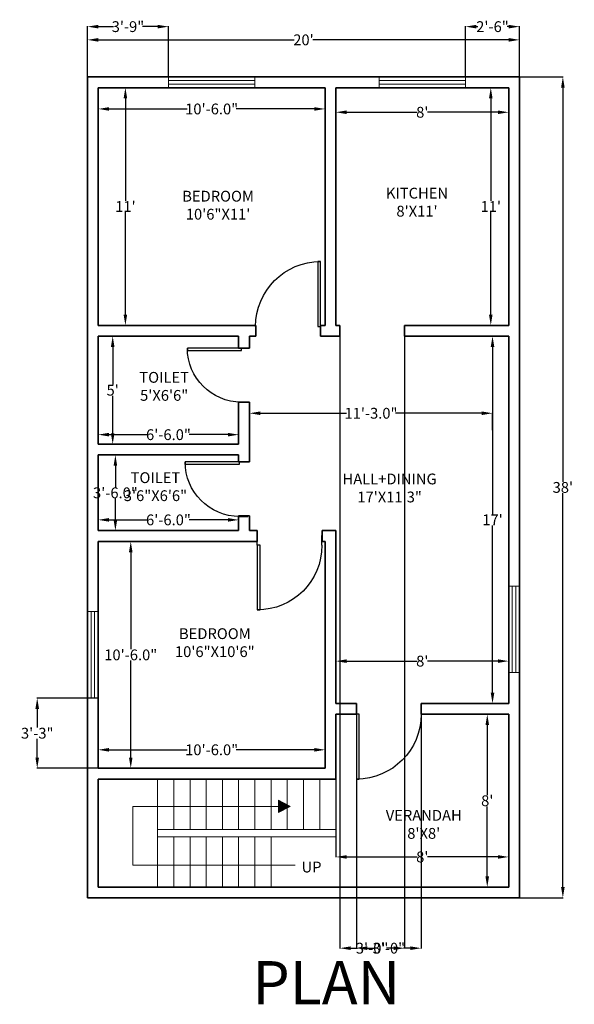
# Model space of a CAD drawing. Units: inches. Extents: x 329 to 1300, y 173 to 760.
# Tile 1 of 3: x 329 to 637, y 214 to 760. Entities that reach past the tile are written whole.
import ezdxf

# ---------------------------------------------------------------- set-up
doc = ezdxf.new("R2010")
doc.units = ezdxf.units.IN
doc.header["$MEASUREMENT"] = 0
doc.layers.add('A-ANNO-PATT', color=251, linetype='Continuous', lineweight=13, true_color=0x636466)
for name, color, linetype, lineweight in [('A-ANNO-SYMB', 7, 'Continuous', 18), ('A-ANNO-TEXT', 7, 'Continuous', 18), ('A-ANNO-TITL', 1, 'Continuous', 25), ('A-AREA-IDEN', 1, 'Continuous', 18), ('A-FLOR-STRS', 7, 'Continuous', 18), ('A-GLAZ', 4, 'Continuous', 18), ('A-WALL', 7, 'Continuous', 35), ('DIMENSION', 80, 'Continuous', 13), ('DOOR', 27, 'Continuous', 25)]:
    doc.layers.add(name, color=color, linetype=linetype, lineweight=lineweight)
doc.styles.get("Standard").update_dxf_attribs({"font": 'arial.ttf'})
doc.dimstyles.get("Standard").update_dxf_attribs({"dimtxt": 6, "dimasz": 6, "dimexe": 0.18, "dimexo": 0.0625, "dimgap": 0.09, "dimtad": 0, "dimtih": 1, "dimtoh": 1, "dimdec": 1, "dimzin": 0, "dimdsep": 46, "dimlunit": 3, "dimtxsty": 'Standard', "dimcen": 0.09, "dimadec": 0, "dimazin": 0, "dimtfac": 1, "dimtdec": 1, "dimtofl": 0, "dimtmove": 0, "dimatfit": 3, "dimfxl": 1, "dimtolj": 1, "dimtzin": 0, "dimarcsym": 0})

# ---------------------------------------------------------------- blocks, each defined once
blk = doc.blocks.new('*U2')
for p, q in [((0, 0), (0, -6)), ((40, 0), (40, -6))]:
    blk.add_line(p, q)
blk.add_lwpolyline([(0, 0), (0, 40), (1.75, 40), (1.75, 0)], close=True)
blk.add_arc((0, 0), 40, 0, 90)
blk = doc.blocks.new('*D22')
at = {"layer": 'Defpoints', "color": 0, "transparency": 16777216}
for p in [(606.67, 749.18), (366.67, 728.62), (606.67, 728.62)]:
    blk.add_point(p, dxfattribs=at)
at = {"layer": 'DIMENSION', "color": 0, "lineweight": -2, "transparency": 16777216}
for p, q in [((366.67, 728.68), (366.67, 749.36)), ((372.67, 749.18), (481.44, 749.18)), ((600.67, 749.18), (491.9, 749.18)), ((606.67, 728.68), (606.67, 749.36))]:
    blk.add_line(p, q, dxfattribs=at)
at = {"layer": 'DIMENSION', "color": 0, "transparency": 16777216}
for points in [[(372.67, 750.18), (372.67, 748.18), (366.67, 749.18)], [(600.67, 750.18), (600.67, 748.18), (606.67, 749.18)]]:
    blk.add_solid(points, dxfattribs=at)
at = {"layer": 'DIMENSION', "color": 0, "transparency": 16777216, "insert": (486.67, 749.18), "char_height": 6, "attachment_point": 5}
blk.add_mtext("\\A1;20'", dxfattribs=at)
blk = doc.blocks.new('*D23')
at = {"layer": 'Defpoints', "color": 0, "transparency": 16777216}
for p in [(606.67, 728.62), (606.67, 272.62), (630.76, 272.62)]:
    blk.add_point(p, dxfattribs=at)
at = {"layer": 'DIMENSION', "color": 0, "lineweight": -2, "transparency": 16777216}
for p, q in [((606.73, 728.62), (630.94, 728.62)), ((630.76, 722.62), (630.76, 503.77)), ((630.76, 278.62), (630.76, 497.46)), ((606.73, 272.62), (630.94, 272.62))]:
    blk.add_line(p, q, dxfattribs=at)
at = {"layer": 'DIMENSION', "color": 0, "transparency": 16777216}
for points in [[(629.76, 722.62), (631.76, 722.62), (630.76, 728.62)], [(629.76, 278.62), (631.76, 278.62), (630.76, 272.62)]]:
    blk.add_solid(points, dxfattribs=at)
at = {"layer": 'DIMENSION', "color": 0, "transparency": 16777216, "insert": (630.76, 500.62), "char_height": 6, "attachment_point": 5}
blk.add_mtext("\\A1;38'", dxfattribs=at)
blk = doc.blocks.new('*D24')
at = {"layer": 'Defpoints', "color": 0, "transparency": 16777216}
for p in [(372.67, 722.62), (372.67, 590.62), (387.75, 590.62)]:
    blk.add_point(p, dxfattribs=at)
at = {"layer": 'DIMENSION', "color": 0, "lineweight": -2, "transparency": 16777216}
for p, q in [((372.73, 722.62), (387.93, 722.62)), ((387.75, 716.62), (387.75, 659.72)), ((387.75, 596.62), (387.75, 653.51)), ((372.73, 590.62), (387.93, 590.62))]:
    blk.add_line(p, q, dxfattribs=at)
at = {"layer": 'DIMENSION', "color": 0, "transparency": 16777216}
for points in [[(386.75, 716.62), (388.75, 716.62), (387.75, 722.62)], [(386.75, 596.62), (388.75, 596.62), (387.75, 590.62)]]:
    blk.add_solid(points, dxfattribs=at)
at = {"layer": 'DIMENSION', "color": 0, "transparency": 16777216, "insert": (387.75, 656.62), "char_height": 6, "attachment_point": 5}
blk.add_mtext("\\A1;11'", dxfattribs=at)
blk = doc.blocks.new('*D25')
at = {"layer": 'Defpoints', "color": 0, "transparency": 16777216}
for p in [(372.67, 722.62), (498.67, 722.62), (498.67, 710.8)]:
    blk.add_point(p, dxfattribs=at)
at = {"layer": 'DIMENSION', "color": 0, "lineweight": -2, "transparency": 16777216}
for p, q in [((372.67, 722.55), (372.67, 710.62)), ((498.67, 722.55), (498.67, 710.62)), ((378.67, 710.8), (422.06, 710.8)), ((492.67, 710.8), (449.28, 710.8))]:
    blk.add_line(p, q, dxfattribs=at)
at = {"layer": 'DIMENSION', "color": 0, "transparency": 16777216}
for points in [[(378.67, 711.8), (378.67, 709.8), (372.67, 710.8)], [(492.67, 711.8), (492.67, 709.8), (498.67, 710.8)]]:
    blk.add_solid(points, dxfattribs=at)
at = {"layer": 'DIMENSION', "color": 0, "transparency": 16777216, "insert": (435.67, 710.8), "char_height": 6, "attachment_point": 5}
blk.add_mtext('\\A1;10\'-6.0"', dxfattribs=at)
blk = doc.blocks.new('*D26')
at = {"layer": 'Defpoints', "color": 0, "transparency": 16777216}
for p in [(600.67, 722.62), (590.73, 590.62), (600.67, 590.62)]:
    blk.add_point(p, dxfattribs=at)
at = {"layer": 'DIMENSION', "color": 0, "lineweight": -2, "transparency": 16777216}
for p, q in [((600.61, 722.62), (590.55, 722.62)), ((590.73, 716.62), (590.73, 659.72)), ((590.73, 596.62), (590.73, 653.51)), ((600.61, 590.62), (590.55, 590.62))]:
    blk.add_line(p, q, dxfattribs=at)
at = {"layer": 'DIMENSION', "color": 0, "transparency": 16777216}
for points in [[(589.73, 716.62), (591.73, 716.62), (590.73, 722.62)], [(589.73, 596.62), (591.73, 596.62), (590.73, 590.62)]]:
    blk.add_solid(points, dxfattribs=at)
at = {"layer": 'DIMENSION', "color": 0, "transparency": 16777216, "insert": (590.73, 656.62), "char_height": 6, "attachment_point": 5}
blk.add_mtext("\\A1;11'", dxfattribs=at)
blk = doc.blocks.new('*D27')
at = {"layer": 'Defpoints', "color": 0, "transparency": 16777216}
for p in [(504.67, 722.62), (600.67, 722.62), (600.67, 708.96)]:
    blk.add_point(p, dxfattribs=at)
at = {"layer": 'DIMENSION', "color": 0, "lineweight": -2, "transparency": 16777216}
for p, q in [((504.67, 722.55), (504.67, 708.78)), ((600.67, 722.55), (600.67, 708.78)), ((510.67, 708.96), (549.82, 708.96)), ((594.67, 708.96), (555.53, 708.96))]:
    blk.add_line(p, q, dxfattribs=at)
at = {"layer": 'DIMENSION', "color": 0, "transparency": 16777216}
for points in [[(510.67, 709.96), (510.67, 707.96), (504.67, 708.96)], [(594.67, 709.96), (594.67, 707.96), (600.67, 708.96)]]:
    blk.add_solid(points, dxfattribs=at)
at = {"layer": 'DIMENSION', "color": 0, "transparency": 16777216, "insert": (552.67, 708.96), "char_height": 6, "attachment_point": 5}
blk.add_mtext("\\A1;8'", dxfattribs=at)
blk = doc.blocks.new('*D28')
at = {"layer": 'Defpoints', "color": 0, "transparency": 16777216}
for p in [(372.67, 584.62), (374.19, 524.62), (380.69, 524.62)]:
    blk.add_point(p, dxfattribs=at)
at = {"layer": 'DIMENSION', "color": 0, "lineweight": -2, "transparency": 16777216}
for p, q in [((372.73, 584.62), (380.87, 584.62)), ((380.69, 578.62), (380.69, 557.76)), ((380.69, 530.62), (380.69, 551.48)), ((374.25, 524.62), (380.87, 524.62))]:
    blk.add_line(p, q, dxfattribs=at)
at = {"layer": 'DIMENSION', "color": 0, "transparency": 16777216}
for points in [[(379.69, 578.62), (381.69, 578.62), (380.69, 584.62)], [(379.69, 530.62), (381.69, 530.62), (380.69, 524.62)]]:
    blk.add_solid(points, dxfattribs=at)
at = {"layer": 'DIMENSION', "color": 0, "transparency": 16777216, "insert": (380.69, 554.62), "char_height": 6, "attachment_point": 5}
blk.add_mtext("\\A1;5'", dxfattribs=at)
blk = doc.blocks.new('*D29')
at = {"layer": 'Defpoints', "color": 0, "transparency": 16777216}
for p in [(450.67, 529.92), (372.67, 524.62), (450.67, 524.62)]:
    blk.add_point(p, dxfattribs=at)
at = {"layer": 'DIMENSION', "color": 0, "lineweight": -2, "transparency": 16777216}
for p, q in [((372.67, 524.68), (372.67, 530.1)), ((378.67, 529.92), (400.09, 529.92)), ((444.67, 529.92), (423.25, 529.92)), ((450.67, 524.68), (450.67, 530.1))]:
    blk.add_line(p, q, dxfattribs=at)
at = {"layer": 'DIMENSION', "color": 0, "transparency": 16777216}
for points in [[(378.67, 530.92), (378.67, 528.92), (372.67, 529.92)], [(444.67, 530.92), (444.67, 528.92), (450.67, 529.92)]]:
    blk.add_solid(points, dxfattribs=at)
at = {"layer": 'DIMENSION', "color": 0, "transparency": 16777216, "insert": (411.67, 529.92), "char_height": 6, "attachment_point": 5}
blk.add_mtext('\\A1;6\'-6.0"', dxfattribs=at)
blk = doc.blocks.new('*D30')
at = {"layer": 'Defpoints', "color": 0, "transparency": 16777216}
for p in [(372.67, 518.62), (372.67, 476.62), (382.2, 476.62)]:
    blk.add_point(p, dxfattribs=at)
at = {"layer": 'DIMENSION', "color": 0, "lineweight": -2, "transparency": 16777216}
for p, q in [((372.73, 518.62), (382.38, 518.62)), ((382.2, 512.62), (382.2, 500.77)), ((382.2, 482.62), (382.2, 494.46)), ((372.73, 476.62), (382.38, 476.62))]:
    blk.add_line(p, q, dxfattribs=at)
at = {"layer": 'DIMENSION', "color": 0, "transparency": 16777216}
for points in [[(381.2, 512.62), (383.2, 512.62), (382.2, 518.62)], [(381.2, 482.62), (383.2, 482.62), (382.2, 476.62)]]:
    blk.add_solid(points, dxfattribs=at)
at = {"layer": 'DIMENSION', "color": 0, "transparency": 16777216, "insert": (382.2, 497.62), "char_height": 6, "attachment_point": 5}
blk.add_mtext('\\A1;3\'-6.0"', dxfattribs=at)
blk = doc.blocks.new('*D31')
at = {"layer": 'Defpoints', "color": 0, "transparency": 16777216}
for p in [(450.67, 482.59), (372.67, 476.62), (450.67, 476.62)]:
    blk.add_point(p, dxfattribs=at)
at = {"layer": 'DIMENSION', "color": 0, "lineweight": -2, "transparency": 16777216}
for p, q in [((372.67, 476.68), (372.67, 482.77)), ((378.67, 482.59), (400.09, 482.59)), ((444.67, 482.59), (423.25, 482.59)), ((450.67, 476.68), (450.67, 482.77))]:
    blk.add_line(p, q, dxfattribs=at)
at = {"layer": 'DIMENSION', "color": 0, "transparency": 16777216}
for points in [[(378.67, 483.59), (378.67, 481.59), (372.67, 482.59)], [(444.67, 483.59), (444.67, 481.59), (450.67, 482.59)]]:
    blk.add_solid(points, dxfattribs=at)
at = {"layer": 'DIMENSION', "color": 0, "transparency": 16777216, "insert": (411.67, 482.59), "char_height": 6, "attachment_point": 5}
blk.add_mtext('\\A1;6\'-6.0"', dxfattribs=at)
blk = doc.blocks.new('*D32')
at = {"layer": 'Defpoints', "color": 0, "transparency": 16777216}
for p in [(498.67, 354.9), (372.67, 344.62), (498.67, 344.62)]:
    blk.add_point(p, dxfattribs=at)
at = {"layer": 'DIMENSION', "color": 0, "lineweight": -2, "transparency": 16777216}
for p, q in [((372.67, 344.68), (372.67, 355.08)), ((378.67, 354.9), (422.06, 354.9)), ((492.67, 354.9), (449.28, 354.9)), ((498.67, 344.68), (498.67, 355.08))]:
    blk.add_line(p, q, dxfattribs=at)
at = {"layer": 'DIMENSION', "color": 0, "transparency": 16777216}
for points in [[(378.67, 355.9), (378.67, 353.9), (372.67, 354.9)], [(492.67, 355.9), (492.67, 353.9), (498.67, 354.9)]]:
    blk.add_solid(points, dxfattribs=at)
at = {"layer": 'DIMENSION', "color": 0, "transparency": 16777216, "insert": (435.67, 354.9), "char_height": 6, "attachment_point": 5}
blk.add_mtext('\\A1;10\'-6.0"', dxfattribs=at)
blk = doc.blocks.new('*D33')
at = {"layer": 'Defpoints', "color": 0, "transparency": 16777216}
for p in [(372.67, 470.62), (390.72, 470.62), (372.67, 344.62)]:
    blk.add_point(p, dxfattribs=at)
at = {"layer": 'DIMENSION', "color": 0, "lineweight": -2, "transparency": 16777216}
for p, q in [((372.73, 470.62), (390.9, 470.62)), ((390.72, 464.62), (390.72, 410.77)), ((390.72, 350.62), (390.72, 404.46)), ((372.73, 344.62), (390.9, 344.62))]:
    blk.add_line(p, q, dxfattribs=at)
at = {"layer": 'DIMENSION', "color": 0, "transparency": 16777216}
for points in [[(389.72, 464.62), (391.72, 464.62), (390.72, 470.62)], [(389.72, 350.62), (391.72, 350.62), (390.72, 344.62)]]:
    blk.add_solid(points, dxfattribs=at)
at = {"layer": 'DIMENSION', "color": 0, "transparency": 16777216, "insert": (390.72, 407.62), "char_height": 6, "attachment_point": 5}
blk.add_mtext('\\A1;10\'-6.0"', dxfattribs=at)
blk = doc.blocks.new('*D34')
at = {"layer": 'Defpoints', "color": 0, "transparency": 16777216}
for p in [(600.67, 584.62), (591.69, 380.62), (600.67, 380.62)]:
    blk.add_point(p, dxfattribs=at)
at = {"layer": 'DIMENSION', "color": 0, "lineweight": -2, "transparency": 16777216}
for p, q in [((600.61, 584.62), (591.51, 584.62)), ((591.69, 578.62), (591.69, 485.72)), ((591.69, 386.62), (591.69, 479.51)), ((600.61, 380.62), (591.51, 380.62))]:
    blk.add_line(p, q, dxfattribs=at)
at = {"layer": 'DIMENSION', "color": 0, "transparency": 16777216}
for points in [[(590.69, 578.62), (592.69, 578.62), (591.69, 584.62)], [(590.69, 386.62), (592.69, 386.62), (591.69, 380.62)]]:
    blk.add_solid(points, dxfattribs=at)
at = {"layer": 'DIMENSION', "color": 0, "transparency": 16777216, "insert": (591.69, 482.62), "char_height": 6, "attachment_point": 5}
blk.add_mtext("\\A1;17'", dxfattribs=at)
blk = doc.blocks.new('*D35')
at = {"layer": 'Defpoints', "color": 0, "transparency": 16777216}
for p in [(591.69, 541.8), (456.67, 532.4), (591.69, 532.4)]:
    blk.add_point(p, dxfattribs=at)
at = {"layer": 'DIMENSION', "color": 0, "lineweight": -2, "transparency": 16777216}
for p, q in [((456.67, 532.47), (456.67, 541.98)), ((462.67, 541.8), (510.57, 541.8)), ((585.69, 541.8), (537.79, 541.8)), ((591.69, 532.47), (591.69, 541.98))]:
    blk.add_line(p, q, dxfattribs=at)
at = {"layer": 'DIMENSION', "color": 0, "transparency": 16777216}
for points in [[(462.67, 542.8), (462.67, 540.8), (456.67, 541.8)], [(585.69, 542.8), (585.69, 540.8), (591.69, 541.8)]]:
    blk.add_solid(points, dxfattribs=at)
at = {"layer": 'DIMENSION', "color": 0, "transparency": 16777216, "insert": (524.18, 541.8), "char_height": 6, "attachment_point": 5}
blk.add_mtext('\\A1;11\'-3.0"', dxfattribs=at)
blk = doc.blocks.new('*D36')
at = {"layer": 'Defpoints', "color": 0, "transparency": 16777216}
for p in [(600.67, 404.14), (504.67, 390.46), (600.67, 390.46)]:
    blk.add_point(p, dxfattribs=at)
at = {"layer": 'DIMENSION', "color": 0, "lineweight": -2, "transparency": 16777216}
for p, q in [((504.67, 390.52), (504.67, 404.32)), ((510.67, 404.14), (549.82, 404.14)), ((594.67, 404.14), (555.53, 404.14)), ((600.67, 390.52), (600.67, 404.32))]:
    blk.add_line(p, q, dxfattribs=at)
at = {"layer": 'DIMENSION', "color": 0, "transparency": 16777216}
for points in [[(510.67, 405.14), (510.67, 403.14), (504.67, 404.14)], [(594.67, 405.14), (594.67, 403.14), (600.67, 404.14)]]:
    blk.add_solid(points, dxfattribs=at)
at = {"layer": 'DIMENSION', "color": 0, "transparency": 16777216, "insert": (552.67, 404.14), "char_height": 6, "attachment_point": 5}
blk.add_mtext("\\A1;8'", dxfattribs=at)
blk = doc.blocks.new('*D37')
at = {"layer": 'Defpoints', "color": 0, "transparency": 16777216}
for p in [(504.67, 338.62), (600.67, 335.99), (600.67, 295.39)]:
    blk.add_point(p, dxfattribs=at)
at = {"layer": 'DIMENSION', "color": 0, "lineweight": -2, "transparency": 16777216}
for p, q in [((504.67, 338.55), (504.67, 295.21)), ((600.67, 335.92), (600.67, 295.21)), ((510.67, 295.39), (549.82, 295.39)), ((594.67, 295.39), (555.53, 295.39))]:
    blk.add_line(p, q, dxfattribs=at)
at = {"layer": 'DIMENSION', "color": 0, "transparency": 16777216}
for points in [[(510.67, 296.39), (510.67, 294.39), (504.67, 295.39)], [(594.67, 296.39), (594.67, 294.39), (600.67, 295.39)]]:
    blk.add_solid(points, dxfattribs=at)
at = {"layer": 'DIMENSION', "color": 0, "transparency": 16777216, "insert": (552.67, 295.39), "char_height": 6, "attachment_point": 5}
blk.add_mtext("\\A1;8'", dxfattribs=at)
blk = doc.blocks.new('*D38')
at = {"layer": 'Defpoints', "color": 0, "transparency": 16777216}
for p in [(600.67, 374.62), (588.77, 278.62), (600.67, 278.62)]:
    blk.add_point(p, dxfattribs=at)
at = {"layer": 'DIMENSION', "color": 0, "lineweight": -2, "transparency": 16777216}
for p, q in [((600.61, 374.62), (588.59, 374.62)), ((588.77, 368.62), (588.77, 329.77)), ((588.77, 284.62), (588.77, 323.46)), ((600.61, 278.62), (588.59, 278.62))]:
    blk.add_line(p, q, dxfattribs=at)
at = {"layer": 'DIMENSION', "color": 0, "transparency": 16777216}
for points in [[(587.77, 368.62), (589.77, 368.62), (588.77, 374.62)], [(587.77, 284.62), (589.77, 284.62), (588.77, 278.62)]]:
    blk.add_solid(points, dxfattribs=at)
at = {"layer": 'DIMENSION', "color": 0, "transparency": 16777216, "insert": (588.77, 326.62), "char_height": 6, "attachment_point": 5}
blk.add_mtext("\\A1;8'", dxfattribs=at)
blk = doc.blocks.new('WIN-W1-48IN')
for p, q in [((0, 0), (0, 6)), ((48, 0), (48, 6)), ((0, 4), (48, 4)), ((0, 2), (48, 2))]:
    blk.add_line(p, q)
blk = doc.blocks.new('*D50')
at = {"layer": 'Defpoints', "color": 0, "transparency": 16777216}
for p in [(411.67, 756.52), (366.67, 728.62), (411.67, 728.62)]:
    blk.add_point(p, dxfattribs=at)
at = {"layer": 'DIMENSION', "color": 0, "lineweight": -2, "transparency": 16777216}
for p, q in [((366.67, 728.68), (366.67, 756.7)), ((372.67, 756.52), (381.11, 756.52)), ((405.67, 756.52), (397.23, 756.52)), ((411.67, 728.68), (411.67, 756.7))]:
    blk.add_line(p, q, dxfattribs=at)
at = {"layer": 'DIMENSION', "color": 0, "transparency": 16777216}
for points in [[(372.67, 757.52), (372.67, 755.52), (366.67, 756.52)], [(405.67, 757.52), (405.67, 755.52), (411.67, 756.52)]]:
    blk.add_solid(points, dxfattribs=at)
at = {"layer": 'DIMENSION', "color": 0, "transparency": 16777216, "insert": (389.17, 756.52), "char_height": 6, "attachment_point": 5}
blk.add_mtext('\\A1;3\'-9"', dxfattribs=at)
blk = doc.blocks.new('*D51')
at = {"layer": 'Defpoints', "color": 0, "transparency": 16777216}
for p in [(606.67, 756.52), (576.67, 728.62), (606.67, 728.62)]:
    blk.add_point(p, dxfattribs=at)
at = {"layer": 'DIMENSION', "color": 0, "lineweight": -2, "transparency": 16777216}
for p, q in [((576.67, 728.68), (576.67, 756.7)), ((582.67, 756.52), (583.56, 756.52)), ((600.67, 756.52), (599.79, 756.52)), ((606.67, 728.68), (606.67, 756.7))]:
    blk.add_line(p, q, dxfattribs=at)
at = {"layer": 'DIMENSION', "color": 0, "transparency": 16777216}
for points in [[(582.67, 757.52), (582.67, 755.52), (576.67, 756.52)], [(600.67, 757.52), (600.67, 755.52), (606.67, 756.52)]]:
    blk.add_solid(points, dxfattribs=at)
at = {"layer": 'DIMENSION', "color": 0, "transparency": 16777216, "insert": (591.67, 756.52), "char_height": 6, "attachment_point": 5}
blk.add_mtext('\\A1;2\'-6"', dxfattribs=at)
blk = doc.blocks.new('*D52')
at = {"layer": 'Defpoints', "color": 0, "transparency": 16777216}
for p in [(338.77, 383.62), (372.67, 383.62), (372.67, 344.62)]:
    blk.add_point(p, dxfattribs=at)
at = {"layer": 'DIMENSION', "color": 0, "lineweight": -2, "transparency": 16777216}
for p, q in [((372.61, 383.62), (338.59, 383.62)), ((338.77, 377.62), (338.77, 367.27)), ((338.77, 350.62), (338.77, 360.96)), ((372.61, 344.62), (338.59, 344.62))]:
    blk.add_line(p, q, dxfattribs=at)
at = {"layer": 'DIMENSION', "color": 0, "transparency": 16777216}
for points in [[(337.77, 377.62), (339.77, 377.62), (338.77, 383.62)], [(337.77, 350.62), (339.77, 350.62), (338.77, 344.62)]]:
    blk.add_solid(points, dxfattribs=at)
at = {"layer": 'DIMENSION', "color": 0, "transparency": 16777216, "insert": (338.77, 364.12), "char_height": 6, "attachment_point": 5}
blk.add_mtext('\\A1;3\'-3"', dxfattribs=at)
blk = doc.blocks.new('*D54')
at = {"layer": 'Defpoints', "color": 0, "transparency": 16777216}
for p in [(516.11, 374.62), (552.07, 374.6), (552.07, 244.72)]:
    blk.add_point(p, dxfattribs=at)
at = {"layer": 'DIMENSION', "color": 0, "lineweight": -2, "transparency": 16777216}
for p, q in [((516.11, 374.55), (516.11, 244.54)), ((552.07, 374.54), (552.07, 244.54)), ((522.11, 244.72), (526.03, 244.72)), ((546.07, 244.72), (542.15, 244.72))]:
    blk.add_line(p, q, dxfattribs=at)
at = {"layer": 'DIMENSION', "color": 0, "transparency": 16777216}
for points in [[(522.11, 245.72), (522.11, 243.72), (516.11, 244.72)], [(546.07, 245.72), (546.07, 243.72), (552.07, 244.72)]]:
    blk.add_solid(points, dxfattribs=at)
at = {"layer": 'DIMENSION', "color": 0, "transparency": 16777216, "insert": (534.09, 244.72), "char_height": 6, "attachment_point": 5}
blk.add_mtext('\\A1;3\'-0"', dxfattribs=at)
blk = doc.blocks.new('*D55')
at = {"layer": 'Defpoints', "color": 0, "transparency": 16777216}
for p in [(506.81, 590.62), (542.81, 590.62), (542.81, 244.72)]:
    blk.add_point(p, dxfattribs=at)
at = {"layer": 'DIMENSION', "color": 0, "lineweight": -2, "transparency": 16777216}
for p, q in [((506.81, 590.55), (506.81, 244.54)), ((542.81, 590.55), (542.81, 244.54)), ((512.81, 244.72), (516.75, 244.72)), ((536.81, 244.72), (532.87, 244.72))]:
    blk.add_line(p, q, dxfattribs=at)
at = {"layer": 'DIMENSION', "color": 0, "transparency": 16777216}
for points in [[(512.81, 245.72), (512.81, 243.72), (506.81, 244.72)], [(536.81, 245.72), (536.81, 243.72), (542.81, 244.72)]]:
    blk.add_solid(points, dxfattribs=at)
at = {"layer": 'DIMENSION', "color": 0, "transparency": 16777216, "insert": (524.81, 244.72), "char_height": 6, "attachment_point": 5}
blk.add_mtext('\\A1;3\'-0"', dxfattribs=at)

msp = doc.modelspace()

# ---------------------------------------------------------------- hatches: boundary and pattern name
at = {"layer": 'A-ANNO-PATT'}
h = msp.add_hatch(dxfattribs=at)
h.set_pattern_fill('ANSI31', color=256)
h.paths.add_polyline_path([(477.67, 324.36), (472.8, 326.94), (472.8, 323.48), (472.8, 320.13), (477.67, 322.63)])
h.paths.add_polyline_path([(479.33, 323.48), (477.67, 324.36), (477.67, 322.63)])
h = msp.add_hatch(color=256, dxfattribs=at)
h.dxf.hatch_style = 1
h.paths.add_polyline_path([(477.67, 324.36), (472.8, 326.94), (472.8, 323.48), (472.8, 320.13), (477.67, 322.63)])
h.paths.add_polyline_path([(477.67, 324.36), (477.67, 322.63), (479.33, 323.48)])

# ---------------------------------------------------------------- linework, layer by layer
at = {"layer": 'A-ANNO-SYMB'}
for p, q in [((391.83, 290.84), (391.83, 323.48)), ((391.83, 323.48), (472.8, 323.48)), ((472.8, 323.48), (472.8, 326.94)), ((472.8, 326.94), (479.33, 323.48)), ((479.33, 323.48), (472.8, 320.13)), ((472.8, 320.13), (472.8, 323.48)), ((481.99, 290.84), (391.83, 290.84))]:
    msp.add_line(p, q, dxfattribs=at)
at = {"layer": 'A-FLOR-STRS'}
for p, q in [((405.67, 338.62), (405.67, 278.62)), ((414.67, 338.62), (414.67, 310.62)), ((423.67, 338.62), (423.67, 310.62)), ((432.67, 338.62), (432.67, 310.62)), ((441.67, 338.62), (441.67, 310.62)), ((450.67, 338.62), (450.67, 310.62)), ((459.67, 338.62), (459.67, 310.62)), ((468.67, 338.62), (468.67, 310.62)), ((477.67, 338.62), (477.67, 324.36)), ((486.67, 338.62), (486.67, 310.62)), ((495.67, 338.62), (495.67, 310.62)), ((504.67, 338.62), (504.67, 306.62)), ((477.67, 322.63), (477.67, 310.62)), ((405.67, 310.62), (504.67, 310.62)), ((405.67, 306.62), (504.67, 306.62)), ((414.67, 306.62), (414.67, 278.62)), ((423.67, 306.62), (423.67, 278.62)), ((432.67, 306.62), (432.67, 278.62)), ((441.67, 306.62), (441.67, 278.62)), ((450.67, 306.62), (450.67, 278.62)), ((459.67, 306.62), (459.67, 278.62)), ((468.67, 306.62), (468.67, 278.62))]:
    msp.add_line(p, q, dxfattribs=at)
at = {"layer": 'A-WALL'}
for p, q in [((606.67, 728.62), (366.67, 728.62)), ((366.67, 728.62), (366.67, 272.62)), ((606.67, 272.62), (606.67, 728.62)), ((372.67, 722.62), (372.67, 590.62)), ((498.67, 722.62), (372.67, 722.62)), ((498.67, 722.62), (498.67, 590.62)), ((600.67, 722.62), (504.67, 722.62)), ((504.67, 722.62), (504.67, 590.62)), ((600.67, 590.62), (600.67, 722.62)), ((460.14, 590.62), (372.67, 590.62)), ((460.14, 590.62), (460.14, 584.62)), ((498.67, 590.62), (496.14, 590.62)), ((496.14, 590.62), (496.14, 584.62)), ((506.81, 590.62), (504.67, 590.62)), ((506.81, 590.62), (506.81, 584.62)), ((600.67, 590.62), (542.81, 590.62)), ((542.81, 590.62), (542.81, 584.62)), ((372.67, 584.62), (372.67, 524.62)), ((450.67, 584.62), (372.67, 584.62)), ((450.67, 584.62), (450.67, 577.98)), ((456.67, 584.62), (456.67, 577.98)), ((460.14, 584.62), (456.67, 584.62)), ((504.67, 584.62), (496.14, 584.62)), ((506.81, 584.62), (504.67, 584.62)), ((600.67, 584.62), (542.81, 584.62)), ((600.67, 380.62), (600.67, 584.62)), ((450.67, 577.98), (456.67, 577.98)), ((450.67, 547.98), (456.67, 547.98)), ((450.67, 547.98), (450.67, 524.62)), ((456.67, 547.98), (456.67, 524.62)), ((450.67, 524.62), (372.67, 524.62)), ((456.67, 524.62), (456.67, 514.8)), ((450.67, 518.62), (372.67, 518.62)), ((372.67, 518.62), (372.67, 476.62)), ((450.67, 518.62), (450.67, 514.8)), ((450.67, 514.8), (456.67, 514.8)), ((450.67, 484.8), (456.67, 484.8)), ((450.67, 484.8), (450.67, 476.62)), ((456.67, 484.8), (456.67, 476.62)), ((450.67, 476.62), (372.67, 476.62)), ((460.98, 476.62), (456.67, 476.62)), ((460.98, 470.62), (460.98, 476.62)), ((504.67, 476.62), (496.98, 476.62)), ((496.98, 470.62), (496.98, 476.62)), ((504.67, 476.62), (504.67, 380.62)), ((372.67, 470.62), (372.67, 344.62)), ((460.98, 470.62), (372.67, 470.62)), ((498.67, 470.62), (496.98, 470.62)), ((498.67, 470.62), (498.67, 344.62)), ((516.11, 380.62), (504.67, 380.62)), ((516.11, 374.62), (516.11, 380.62)), ((600.67, 380.62), (552.11, 380.62)), ((552.11, 374.62), (552.11, 380.62)), ((504.67, 374.62), (504.67, 338.62)), ((516.11, 374.62), (504.67, 374.62)), ((600.67, 374.62), (552.11, 374.62)), ((600.67, 278.62), (600.67, 374.62)), ((498.67, 344.62), (372.67, 344.62)), ((504.67, 338.62), (372.67, 338.62)), ((372.67, 338.62), (372.67, 278.62)), ((372.67, 278.62), (600.67, 278.62)), ((366.67, 272.62), (606.67, 272.62))]:
    msp.add_line(p, q, dxfattribs=at)

# ---------------------------------------------------------------- block references
at = {"layer": 'A-GLAZ'}
msp.add_blockref('WIN-W1-48IN', (411.67, 722.62), dxfattribs=at)
for p, rotation in [((576.67, 728.62), 180), ((600.67, 445.84), 270), ((366.67, 431.62), 270.0000000000003)]:
    msp.add_blockref('WIN-W1-48IN', p, dxfattribs=dict(at, rotation=rotation))
at = {"layer": 'DOOR', "xscale": -0.9012848244184455, "yscale": 0.9012848244184455, "zscale": 0.9012848244184455}
msp.add_blockref('*U2', (496.14, 590.02), dxfattribs=at)
at = {"layer": 'DOOR'}
for p, xscale, yscale, zscale, rotation in [((452.17, 577.98), -0.7497467609316112, 0.7497467609316112, 0.7497467609316112, 90), ((451.21, 514.8), -0.7577850931716829, 0.7577850931716829, 0.7577850931716829, 90), ((460.98, 468.52), -0.8991931185370194, 0.8991931185370194, 0.8991931185370194, 180), ((516.11, 374.6), -0.8991931185370194, 0.8991931185370194, 0.8991931185370194, 180)]:
    msp.add_blockref('*U2', p, dxfattribs=dict(at, xscale=xscale, yscale=yscale, zscale=zscale, rotation=rotation))

# ---------------------------------------------------------------- texts
at = {"layer": 'A-ANNO-TEXT', "insert": (491.16, 292.77), "char_height": 6, "attachment_point": 2}
msp.add_mtext_dynamic_manual_height_columns('UP', width=11.8553, gutter_width=1, heights=[0], dxfattribs=at)
at = {"layer": 'A-ANNO-TITL', "insert": (499.37, 237.55), "char_height": 24, "attachment_point": 2}
msp.add_mtext_dynamic_manual_height_columns('PLAN', width=54.312, gutter_width=1, heights=[16.23], dxfattribs=at)
at = {"layer": 'A-AREA-IDEN', "char_height": 6, "attachment_point": 2}
for s, insert in [("KITCHEN\\P8'X11'", (549.74, 667.03)), ('BEDROOM\\P10\'6"X11\'', (439.24, 665.35)), ('TOILET\\P5\'X6\'6"', (409.28, 564.73)), ('TOILET\\P3\'6"X6\'6"', (404.44, 509.03)), ('HALL+DINING\\P17\'X11\'3"', (534.52, 508.3)), ('BEDROOM\\P10\'6"X10\'6"', (437.42, 422.4)), ("VERANDAH\\P8'X8'", (553.49, 321.48))]:
    msp.add_mtext_dynamic_manual_height_columns(s, width=52.264, gutter_width=1, heights=[0], dxfattribs=dict(at, insert=insert))

# ---------------------------------------------------------------- dimensions: what is measured, and where the dimension line sits
at = {"layer": 'DIMENSION'}
for base, p1, p2, override, picture, middle in [((411.67, 756.52), (366.67, 728.62), (411.67, 728.62), {"dimdec": 1, "dimlfac": 1, "dimrnd": 0, "dimzin": 1, "dimdsep": 46, "dimlunit": 4, "dimfrac": 2}, '*D50', (389.17, 756.52)), ((606.67, 756.52), (576.67, 728.62), (606.67, 728.62), {"dimdec": 1, "dimlfac": 1, "dimrnd": 0, "dimzin": 1, "dimdsep": 46, "dimlunit": 4, "dimfrac": 2}, '*D51', (591.67, 756.52)), ((606.67, 749.18), (366.67, 728.62), (606.67, 728.62), {"dimclrd": 0, "dimclre": 0, "dimclrt": 0}, '*D22', (486.67, 749.18)), ((498.67, 710.8), (372.67, 722.62), (498.67, 722.62), {"dimclrd": 0, "dimclre": 0, "dimclrt": 0}, '*D25', (435.67, 710.8)), ((600.67, 708.96), (504.67, 722.62), (600.67, 722.62), {"dimclrd": 0, "dimclre": 0, "dimclrt": 0}, '*D27', (552.67, 708.96)), ((542.81, 244.72), (506.81, 590.62), (542.81, 590.62), {"dimdec": 1, "dimlfac": 1, "dimrnd": 0, "dimzin": 1, "dimdsep": 46, "dimlunit": 4, "dimfrac": 2}, '*D55', (524.81, 244.72)), ((591.69, 541.8), (456.67, 532.4), (591.69, 532.4), {"dimclrd": 0, "dimclre": 0, "dimclrt": 0}, '*D35', (524.18, 541.8)), ((450.67, 529.92), (372.67, 524.62), (450.67, 524.62), {"dimclrd": 0, "dimclre": 0, "dimclrt": 0}, '*D29', (411.67, 529.92)), ((450.67, 482.59), (372.67, 476.62), (450.67, 476.62), {"dimclrd": 0, "dimclre": 0, "dimclrt": 0}, '*D31', (411.67, 482.59)), ((600.67, 404.14), (504.67, 390.46), (600.67, 390.46), {"dimclrd": 0, "dimclre": 0, "dimclrt": 0}, '*D36', (552.67, 404.14)), ((552.07, 244.72), (516.11, 374.62), (552.07, 374.6), {"dimdec": 1, "dimlfac": 1, "dimrnd": 0, "dimzin": 1, "dimdsep": 46, "dimlunit": 4, "dimfrac": 2}, '*D54', (534.09, 244.72)), ((498.67, 354.9), (372.67, 344.62), (498.67, 344.62), {"dimclrd": 0, "dimclre": 0, "dimclrt": 0}, '*D32', (435.67, 354.9)), ((600.67, 295.39), (504.67, 338.62), (600.67, 335.99), {"dimclrd": 0, "dimclre": 0, "dimclrt": 0}, '*D37', (552.67, 295.39))]:
    dim = msp.add_linear_dim(base=base, p1=p1, p2=p2, dimstyle='Standard', override=override, dxfattribs=at)
    dim.commit()
    dim.dimension.update_dxf_attribs({"geometry": picture, "text_midpoint": middle})
for base, p1, p2, override, picture, middle in [((630.76, 272.62), (606.67, 728.62), (606.67, 272.62), {"dimclrd": 0, "dimclre": 0, "dimclrt": 0}, '*D23', (630.76, 500.62)), ((387.75, 590.62), (372.67, 722.62), (372.67, 590.62), {"dimclrd": 0, "dimclre": 0, "dimclrt": 0}, '*D24', (387.75, 656.62)), ((590.73, 590.62), (600.67, 722.62), (600.67, 590.62), {"dimclrd": 0, "dimclre": 0, "dimclrt": 0}, '*D26', (590.73, 656.62)), ((380.69, 524.62), (372.67, 584.62), (374.19, 524.62), {"dimclrd": 0, "dimclre": 0, "dimclrt": 0}, '*D28', (380.69, 554.62)), ((591.69, 380.62), (600.67, 584.62), (600.67, 380.62), {"dimclrd": 0, "dimclre": 0, "dimclrt": 0}, '*D34', (591.69, 482.62)), ((382.2, 476.62), (372.67, 518.62), (372.67, 476.62), {"dimclrd": 0, "dimclre": 0, "dimclrt": 0}, '*D30', (382.2, 497.62)), ((390.72, 470.62), (372.67, 344.62), (372.67, 470.62), {"dimclrd": 0, "dimclre": 0, "dimclrt": 0}, '*D33', (390.72, 407.62)), ((338.77, 383.62), (372.67, 344.62), (372.67, 383.62), {"dimdec": 1, "dimlfac": 1, "dimrnd": 0, "dimzin": 1, "dimdsep": 46, "dimlunit": 4, "dimfrac": 2}, '*D52', (338.77, 364.12)), ((588.77, 278.62), (600.67, 374.62), (600.67, 278.62), {"dimclrd": 0, "dimclre": 0, "dimclrt": 0}, '*D38', (588.77, 326.62))]:
    dim = msp.add_linear_dim(base=base, p1=p1, p2=p2, angle=90, dimstyle='Standard', override=override, dxfattribs=at)
    dim.commit()
    dim.dimension.update_dxf_attribs({"geometry": picture, "text_midpoint": middle})

doc.saveas('drawing.dxf')
